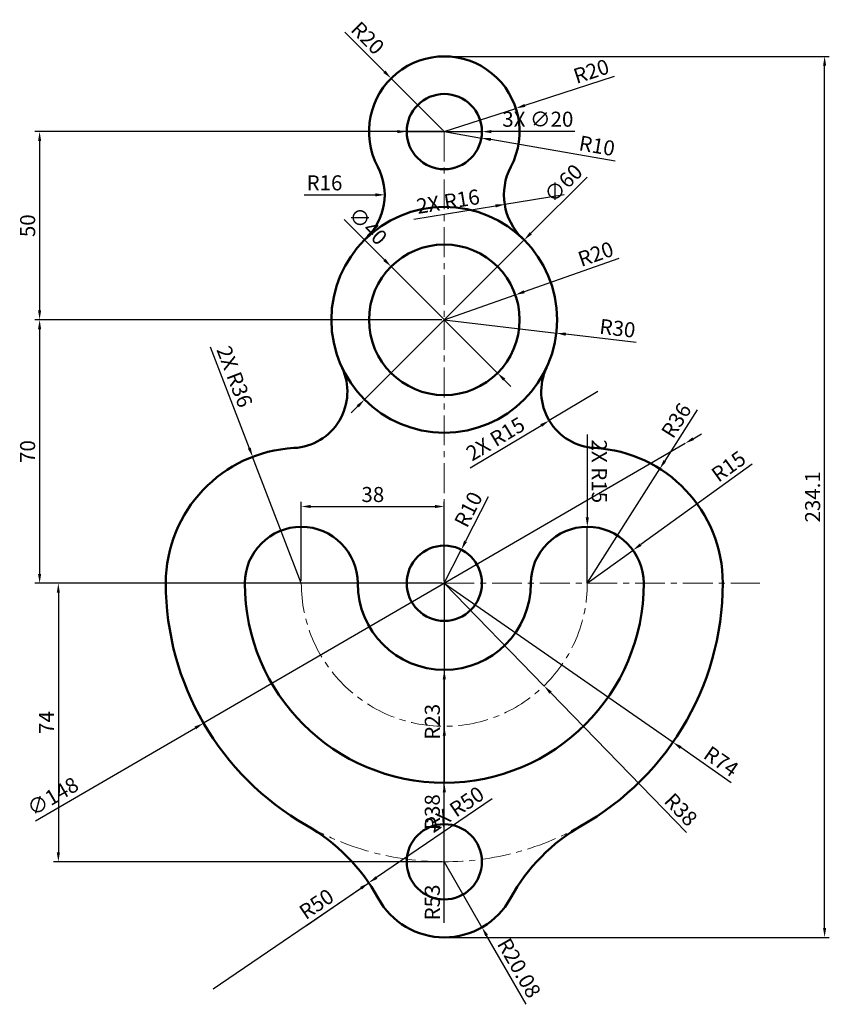
# Model space of a CAD drawing. Units: millimetres. Extents: x 2943 to 3158, y 1764 to 2026.
import ezdxf

# ---------------------------------------------------------------- set-up
doc = ezdxf.new("R2010")
doc.units = ezdxf.units.MM
doc.linetypes.add('CENTER', pattern=[50.8, 31.75, -6.35, 6.35, -6.35])
for name, color, linetype, lineweight in [('M-CNTR', 4, 'CENTER', 18), ('M-DIMS', 2, 'Continuous', 25), ('M-OUTL', 7, 'Continuous', 50)]:
    doc.layers.add(name, color=color, linetype=linetype, lineweight=lineweight)
doc.styles.get("Standard").update_dxf_attribs({"font": 'arial.ttf'})
doc.dimstyles.new('ISO-25', dxfattribs={"dimtxt": 4, "dimasz": 2.5, "dimexe": 1.25, "dimexo": 0.625, "dimtad": 1, "dimtxsty": 'Standard', "dimcen": 2.5, "dimadec": 0, "dimazin": 0, "dimtfac": 1, "dimtmove": 0, "dimatfit": 3, "dimfxl": 1, "dimarcsym": 0})

# ---------------------------------------------------------------- blocks, each defined once
blk = doc.blocks.new('*D1')
at = {"layer": 'Defpoints', "color": 0, "transparency": 16777216}
for p in [(3055.79, 1995.84), (2948.25, 1945.84), (3055.79, 1945.84)]:
    blk.add_point(p, dxfattribs=at)
at = {"layer": 'M-DIMS', "color": 0, "lineweight": -2, "transparency": 16777216}
for p, q in [((3055.16, 1995.84), (2947, 1995.84)), ((2948.25, 1993.34), (2948.25, 1948.34)), ((3055.16, 1945.84), (2947, 1945.84))]:
    blk.add_line(p, q, dxfattribs=at)
at = {"layer": 'M-DIMS', "color": 0, "transparency": 16777216}
for points in [[(2947.83, 1993.34), (2948.66, 1993.34), (2948.25, 1995.84)], [(2947.83, 1948.34), (2948.66, 1948.34), (2948.25, 1945.84)]]:
    blk.add_solid(points, dxfattribs=at)
at = {"layer": 'M-DIMS', "color": 0, "transparency": 16777216, "insert": (2945.58, 1970.84), "char_height": 4, "attachment_point": 5, "rotation": 90}
blk.add_mtext('50', dxfattribs=at)
blk = doc.blocks.new('*D2')
at = {"layer": 'Defpoints', "color": 0, "transparency": 16777216}
for p in [(3055.79, 1945.84), (2948.25, 1875.84), (3055.79, 1875.84)]:
    blk.add_point(p, dxfattribs=at)
at = {"layer": 'M-DIMS', "color": 0, "lineweight": -2, "transparency": 16777216}
for p, q in [((3055.16, 1945.84), (2947, 1945.84)), ((2948.25, 1943.34), (2948.25, 1878.34)), ((3055.16, 1875.84), (2947, 1875.84))]:
    blk.add_line(p, q, dxfattribs=at)
at = {"layer": 'M-DIMS', "color": 0, "transparency": 16777216}
for points in [[(2947.83, 1943.34), (2948.66, 1943.34), (2948.25, 1945.84)], [(2947.83, 1878.34), (2948.66, 1878.34), (2948.25, 1875.84)]]:
    blk.add_solid(points, dxfattribs=at)
at = {"layer": 'M-DIMS', "color": 0, "transparency": 16777216, "insert": (2945.58, 1910.84), "char_height": 4, "attachment_point": 5, "rotation": 90}
blk.add_mtext('70', dxfattribs=at)
blk = doc.blocks.new('*D3')
at = {"layer": 'Defpoints', "color": 0, "transparency": 16777216}
for p in [(3055.79, 1875.84), (2953.23, 1801.84), (3055.79, 1801.84)]:
    blk.add_point(p, dxfattribs=at)
at = {"layer": 'M-DIMS', "color": 0, "lineweight": -2, "transparency": 16777216}
for p, q in [((3055.16, 1875.84), (2951.98, 1875.84)), ((2953.23, 1873.34), (2953.23, 1804.34)), ((3055.16, 1801.84), (2951.98, 1801.84))]:
    blk.add_line(p, q, dxfattribs=at)
at = {"layer": 'M-DIMS', "color": 0, "transparency": 16777216}
for points in [[(2952.81, 1873.34), (2953.64, 1873.34), (2953.23, 1875.84)], [(2952.81, 1804.34), (2953.64, 1804.34), (2953.23, 1801.84)]]:
    blk.add_solid(points, dxfattribs=at)
at = {"layer": 'M-DIMS', "color": 0, "transparency": 16777216, "insert": (2950.6, 1838.84), "char_height": 4, "attachment_point": 5, "rotation": 90}
blk.add_mtext('74', dxfattribs=at)
blk = doc.blocks.new('*D4')
at = {"layer": 'Defpoints', "color": 0, "transparency": 16777216}
for p in [(3055.79, 1896.24), (3017.79, 1875.84), (3055.79, 1875.84)]:
    blk.add_point(p, dxfattribs=at)
at = {"layer": 'M-DIMS', "color": 0, "lineweight": -2, "transparency": 16777216}
for p, q in [((3017.79, 1876.47), (3017.79, 1897.49)), ((3055.79, 1876.47), (3055.79, 1897.49)), ((3020.29, 1896.24), (3053.29, 1896.24))]:
    blk.add_line(p, q, dxfattribs=at)
at = {"layer": 'M-DIMS', "color": 0, "transparency": 16777216}
for points in [[(3020.29, 1896.66), (3020.29, 1895.83), (3017.79, 1896.24)], [(3053.29, 1896.66), (3053.29, 1895.83), (3055.79, 1896.24)]]:
    blk.add_solid(points, dxfattribs=at)
at = {"layer": 'M-DIMS', "color": 0, "transparency": 16777216, "insert": (3036.79, 1898.91), "char_height": 4, "attachment_point": 5}
blk.add_mtext('38', dxfattribs=at)
blk = doc.blocks.new('*D5')
at = {"layer": 'Defpoints', "color": 0, "transparency": 16777216}
for p in [(3074.81, 2002.02), (3055.79, 1995.84)]:
    blk.add_point(p, dxfattribs=at)
at = {"layer": 'M-DIMS', "color": 0, "lineweight": -2, "transparency": 16777216}
for p, q in [((3100.96, 2010.52), (3077.19, 2002.79)), ((3055.79, 1995.84), (3074.81, 2002.02))]:
    blk.add_line(p, q, dxfattribs=at)
at = {"layer": 'M-DIMS', "color": 0, "transparency": 16777216}
blk.add_solid([(3077.06, 2003.19), (3077.32, 2002.4), (3074.81, 2002.02)], dxfattribs=at)
at = {"layer": 'M-DIMS', "color": 0, "transparency": 16777216, "insert": (3095, 2011.39), "char_height": 4, "attachment_point": 5, "rotation": 17.9978}
blk.add_mtext('R20', dxfattribs=at)
blk = doc.blocks.new('*D6')
at = {"layer": 'Defpoints', "color": 0, "transparency": 16777216}
for p in [(3055.79, 1995.84), (3065.64, 1994.14)]:
    blk.add_point(p, dxfattribs=at)
at = {"layer": 'M-DIMS', "color": 0, "lineweight": -2, "transparency": 16777216}
for p, q in [((3055.79, 1995.84), (3065.64, 1994.14)), ((3101.15, 1988.02), (3068.11, 1993.72))]:
    blk.add_line(p, q, dxfattribs=at)
at = {"layer": 'M-DIMS', "color": 0, "transparency": 16777216}
blk.add_solid([(3068.18, 1994.13), (3068.04, 1993.31), (3065.64, 1994.14)], dxfattribs=at)
at = {"layer": 'M-DIMS', "color": 0, "transparency": 16777216, "insert": (3096.28, 1991.57), "char_height": 4, "attachment_point": 5, "rotation": 350.2218}
blk.add_mtext('R10', dxfattribs=at)
blk = doc.blocks.new('*D7')
at = {"layer": 'Defpoints', "color": 0, "transparency": 16777216}
for p in [(3023.95, 1979.04), (3039.95, 1979.04)]:
    blk.add_point(p, dxfattribs=at)
at = {"layer": 'M-DIMS', "color": 0, "lineweight": -2, "transparency": 16777216}
blk.add_line((3018.55, 1979.04), (3037.45, 1979.04), dxfattribs=at)
at = {"layer": 'M-DIMS', "color": 0, "transparency": 16777216}
blk.add_solid([(3037.45, 1979.46), (3037.45, 1978.62), (3039.95, 1979.04)], dxfattribs=at)
at = {"layer": 'M-DIMS', "color": 0, "transparency": 16777216, "insert": (3023.95, 1981.71), "char_height": 4, "attachment_point": 5}
blk.add_mtext('R16', dxfattribs=at)
blk = doc.blocks.new('*D8')
at = {"layer": 'Defpoints', "color": 0, "transparency": 16777216}
for p in [(3060.31, 1884.76), (3055.79, 1875.84)]:
    blk.add_point(p, dxfattribs=at)
at = {"layer": 'M-DIMS', "color": 0, "lineweight": -2, "transparency": 16777216}
for p, q in [((3067.46, 1898.85), (3061.44, 1886.99)), ((3055.79, 1875.84), (3060.31, 1884.76))]:
    blk.add_line(p, q, dxfattribs=at)
at = {"layer": 'M-DIMS', "color": 0, "transparency": 16777216}
blk.add_solid([(3061.07, 1887.18), (3061.81, 1886.8), (3060.31, 1884.76)], dxfattribs=at)
at = {"layer": 'M-DIMS', "color": 0, "transparency": 16777216, "insert": (3062.64, 1895.24), "char_height": 4, "attachment_point": 5, "rotation": 63.1082}
blk.add_mtext('R10', dxfattribs=at)
blk = doc.blocks.new('*D9')
at = {"layer": 'Defpoints', "color": 0, "transparency": 16777216}
for p in [(3105.94, 1884.63), (3093.79, 1875.84)]:
    blk.add_point(p, dxfattribs=at)
at = {"layer": 'M-DIMS', "color": 0, "lineweight": -2, "transparency": 16777216}
for p, q in [((3137.58, 1907.51), (3107.97, 1886.1)), ((3093.79, 1875.84), (3105.94, 1884.63))]:
    blk.add_line(p, q, dxfattribs=at)
at = {"layer": 'M-DIMS', "color": 0, "transparency": 16777216}
blk.add_solid([(3107.73, 1886.43), (3108.21, 1885.76), (3105.94, 1884.63)], dxfattribs=at)
at = {"layer": 'M-DIMS', "color": 0, "transparency": 16777216, "insert": (3131.63, 1906.49), "char_height": 4, "attachment_point": 5, "rotation": 35.8697}
blk.add_mtext('R15', dxfattribs=at)
blk = doc.blocks.new('*D10')
at = {"layer": 'Defpoints', "color": 0, "transparency": 16777216}
for p in [(3113.05, 1906.25), (3093.79, 1875.84)]:
    blk.add_point(p, dxfattribs=at)
at = {"layer": 'M-DIMS', "color": 0, "lineweight": -2, "transparency": 16777216}
for p, q in [((3123.01, 1921.96), (3114.39, 1908.36)), ((3093.79, 1875.84), (3113.05, 1906.25))]:
    blk.add_line(p, q, dxfattribs=at)
at = {"layer": 'M-DIMS', "color": 0, "transparency": 16777216}
blk.add_solid([(3114.04, 1908.59), (3114.74, 1908.14), (3113.05, 1906.25)], dxfattribs=at)
at = {"layer": 'M-DIMS', "color": 0, "transparency": 16777216, "insert": (3117.86, 1918.82), "char_height": 4, "attachment_point": 5, "rotation": 57.646}
blk.add_mtext('R36', dxfattribs=at)
blk = doc.blocks.new('*D11')
at = {"layer": 'Defpoints', "color": 0, "transparency": 16777216}
for p in [(3074.66, 1952.46), (3055.79, 1945.84)]:
    blk.add_point(p, dxfattribs=at)
at = {"layer": 'M-DIMS', "color": 0, "lineweight": -2, "transparency": 16777216}
for p, q in [((3102.17, 1962.11), (3077.02, 1953.29)), ((3055.79, 1945.84), (3074.66, 1952.46))]:
    blk.add_line(p, q, dxfattribs=at)
at = {"layer": 'M-DIMS', "color": 0, "transparency": 16777216}
blk.add_solid([(3076.88, 1953.68), (3077.16, 1952.9), (3074.66, 1952.46)], dxfattribs=at)
at = {"layer": 'M-DIMS', "color": 0, "transparency": 16777216, "insert": (3096.19, 1962.84), "char_height": 4, "attachment_point": 5, "rotation": 19.3299}
blk.add_mtext('R20', dxfattribs=at)
blk = doc.blocks.new('*D12')
at = {"layer": 'Defpoints', "color": 0, "transparency": 16777216}
for p in [(3055.79, 1945.84), (3085.58, 1942.3)]:
    blk.add_point(p, dxfattribs=at)
at = {"layer": 'M-DIMS', "color": 0, "lineweight": -2, "transparency": 16777216}
for p, q in [((3055.79, 1945.84), (3085.58, 1942.3)), ((3106.79, 1939.78), (3088.06, 1942))]:
    blk.add_line(p, q, dxfattribs=at)
at = {"layer": 'M-DIMS', "color": 0, "transparency": 16777216}
blk.add_solid([(3088.11, 1942.42), (3088.01, 1941.59), (3085.58, 1942.3)], dxfattribs=at)
at = {"layer": 'M-DIMS', "color": 0, "transparency": 16777216, "insert": (3101.75, 1943.07), "char_height": 4, "attachment_point": 5, "rotation": 353.2204}
blk.add_mtext('R30', dxfattribs=at)
blk = doc.blocks.new('*D13')
at = {"layer": 'Defpoints', "color": 0, "transparency": 16777216}
for p in [(3055.79, 1875.84), (3082.27, 1848.59)]:
    blk.add_point(p, dxfattribs=at)
at = {"layer": 'M-DIMS', "color": 0, "lineweight": -2, "transparency": 16777216}
for p, q in [((3055.79, 1875.84), (3082.27, 1848.59)), ((3120.15, 1809.62), (3084.02, 1846.8))]:
    blk.add_line(p, q, dxfattribs=at)
at = {"layer": 'M-DIMS', "color": 0, "transparency": 16777216}
blk.add_solid([(3084.31, 1847.09), (3083.72, 1846.51), (3082.27, 1848.59)], dxfattribs=at)
at = {"layer": 'M-DIMS', "color": 0, "transparency": 16777216, "insert": (3118.29, 1815.36), "char_height": 4, "attachment_point": 5, "rotation": 314.1837}
blk.add_mtext('R38', dxfattribs=at)
blk = doc.blocks.new('*D14')
at = {"layer": 'Defpoints', "color": 0, "transparency": 16777216}
for p in [(3055.79, 1875.84), (3116.56, 1833.61)]:
    blk.add_point(p, dxfattribs=at)
at = {"layer": 'M-DIMS', "color": 0, "lineweight": -2, "transparency": 16777216}
for p, q in [((3055.79, 1875.84), (3116.56, 1833.61)), ((3132.02, 1822.86), (3118.61, 1832.18))]:
    blk.add_line(p, q, dxfattribs=at)
at = {"layer": 'M-DIMS', "color": 0, "transparency": 16777216}
blk.add_solid([(3118.85, 1832.53), (3118.37, 1831.84), (3116.56, 1833.61)], dxfattribs=at)
at = {"layer": 'M-DIMS', "color": 0, "transparency": 16777216, "insert": (3129.08, 1828.1), "char_height": 4, "attachment_point": 5, "rotation": 325.2015}
blk.add_mtext('R74', dxfattribs=at)
blk = doc.blocks.new('*D15')
at = {"layer": 'Defpoints', "color": 0, "transparency": 16777216}
for p in [(3035.71, 1796.23), (2994.35, 1768.13)]:
    blk.add_point(p, dxfattribs=at)
at = {"layer": 'M-DIMS', "color": 0, "lineweight": -2, "transparency": 16777216}
blk.add_line((3019.13, 1784.96), (3033.64, 1794.82), dxfattribs=at)
at = {"layer": 'M-DIMS', "color": 0, "transparency": 16777216}
blk.add_solid([(3033.41, 1795.17), (3033.88, 1794.48), (3035.71, 1796.23)], dxfattribs=at)
at = {"layer": 'M-DIMS', "color": 0, "transparency": 16777216, "insert": (3022.1, 1790.2), "char_height": 4, "attachment_point": 5, "rotation": 34.1854}
blk.add_mtext('R50', dxfattribs=at)
blk = doc.blocks.new('HOLE-D20')
blk.add_circle((10, 10), 10)
blk = doc.blocks.new('*D17')
at = {"layer": 'Defpoints', "color": 0, "transparency": 16777216}
for p in [(3055.79, 2015.84), (3156.85, 2015.84), (3055.79, 1781.76)]:
    blk.add_point(p, dxfattribs=at)
at = {"layer": 'M-DIMS', "color": 0, "lineweight": -2, "transparency": 16777216}
for p, q in [((3056.41, 2015.84), (3158.1, 2015.84)), ((3156.85, 1784.26), (3156.85, 2013.34)), ((3056.41, 1781.76), (3158.1, 1781.76))]:
    blk.add_line(p, q, dxfattribs=at)
at = {"layer": 'M-DIMS', "color": 0, "transparency": 16777216}
for points in [[(3156.43, 2013.34), (3157.26, 2013.34), (3156.85, 2015.84)], [(3156.43, 1784.26), (3157.26, 1784.26), (3156.85, 1781.76)]]:
    blk.add_solid(points, dxfattribs=at)
at = {"layer": 'M-DIMS', "color": 0, "transparency": 16777216, "insert": (3154.18, 1898.8), "char_height": 4, "attachment_point": 5, "rotation": 90}
blk.add_mtext('234.1', dxfattribs=at)
blk = doc.blocks.new('*D18')
at = {"layer": 'Defpoints', "color": 0, "transparency": 16777216}
for p in [(3041.65, 2009.98), (3055.79, 1995.84)]:
    blk.add_point(p, dxfattribs=at)
at = {"layer": 'M-DIMS', "color": 0, "lineweight": -2, "transparency": 16777216}
for p, q in [((3029.34, 2022.28), (3039.88, 2011.75)), ((3055.79, 1995.84), (3041.65, 2009.98))]:
    blk.add_line(p, q, dxfattribs=at)
at = {"layer": 'M-DIMS', "color": 0, "transparency": 16777216}
blk.add_solid([(3040.17, 2012.05), (3039.58, 2011.46), (3041.65, 2009.98)], dxfattribs=at)
at = {"layer": 'M-DIMS', "color": 0, "transparency": 16777216, "insert": (3035.05, 2020.35), "char_height": 4, "attachment_point": 5, "rotation": 315.0007}
blk.add_mtext('R20', dxfattribs=at)
blk = doc.blocks.new('*D19')
at = {"layer": 'Defpoints', "color": 0, "transparency": 16777216}
for p in [(3045.79, 1995.84), (3065.79, 1995.84)]:
    blk.add_point(p, dxfattribs=at)
at = {"layer": 'M-DIMS', "color": 0, "lineweight": -2, "transparency": 16777216}
for p, q in [((3043.29, 1995.84), (3040.79, 1995.84)), ((3045.79, 1995.84), (3065.79, 1995.84)), ((3090.49, 1995.84), (3068.29, 1995.84))]:
    blk.add_line(p, q, dxfattribs=at)
at = {"layer": 'M-DIMS', "color": 0, "transparency": 16777216}
for points in [[(3043.29, 1996.26), (3043.29, 1995.42), (3045.79, 1995.84)], [(3068.29, 1996.26), (3068.29, 1995.42), (3065.79, 1995.84)]]:
    blk.add_solid(points, dxfattribs=at)
at = {"layer": 'M-DIMS', "color": 0, "transparency": 16777216, "insert": (3080.64, 1998.62), "char_height": 4, "attachment_point": 5, "rotation": 359.9986}
blk.add_mtext('3X ∅20', dxfattribs=at)
blk = doc.blocks.new('*D20')
at = {"layer": 'Defpoints', "color": 0, "transparency": 16777216}
for p in [(3087.63, 1979.04), (3071.83, 1976.49)]:
    blk.add_point(p, dxfattribs=at)
at = {"layer": 'M-DIMS', "color": 0, "lineweight": -2, "transparency": 16777216}
for p, q in [((3087.63, 1979.04), (3071.83, 1976.49)), ((3047.68, 1972.58), (3069.37, 1976.09))]:
    blk.add_line(p, q, dxfattribs=at)
at = {"layer": 'M-DIMS', "color": 0, "transparency": 16777216}
blk.add_solid([(3069.3, 1976.5), (3069.43, 1975.68), (3071.83, 1976.49)], dxfattribs=at)
at = {"layer": 'M-DIMS', "color": 0, "transparency": 16777216, "insert": (3056.86, 1976.77), "char_height": 4, "attachment_point": 5, "rotation": 9.1897}
blk.add_mtext('2X R16', dxfattribs=at)
blk = doc.blocks.new('*D21')
at = {"layer": 'Defpoints', "color": 0, "transparency": 16777216}
for p in [(3077, 1967.05), (3034.57, 1924.63)]:
    blk.add_point(p, dxfattribs=at)
at = {"layer": 'M-DIMS', "color": 0, "lineweight": -2, "transparency": 16777216}
for p, q in [((3093.73, 1983.78), (3078.77, 1968.82)), ((3034.57, 1924.63), (3077, 1967.05)), ((3032.81, 1922.86), (3031.04, 1921.09))]:
    blk.add_line(p, q, dxfattribs=at)
at = {"layer": 'M-DIMS', "color": 0, "transparency": 16777216}
for points in [[(3078.48, 1969.12), (3079.07, 1968.53), (3077, 1967.05)], [(3032.51, 1923.16), (3033.1, 1922.57), (3034.57, 1924.63)]]:
    blk.add_solid(points, dxfattribs=at)
at = {"layer": 'M-DIMS', "color": 0, "transparency": 16777216, "insert": (3087.77, 1981.75), "char_height": 4, "attachment_point": 5, "rotation": 44.9971}
blk.add_mtext('∅60', dxfattribs=at)
blk = doc.blocks.new('*D22')
at = {"layer": 'Defpoints', "color": 0, "transparency": 16777216}
for p in [(3041.65, 1959.98), (3069.93, 1931.7)]:
    blk.add_point(p, dxfattribs=at)
at = {"layer": 'M-DIMS', "color": 0, "lineweight": -2, "transparency": 16777216}
for p, q in [((3029.16, 1972.47), (3039.88, 1961.75)), ((3069.93, 1931.7), (3041.65, 1959.98)), ((3071.7, 1929.93), (3073.47, 1928.16))]:
    blk.add_line(p, q, dxfattribs=at)
at = {"layer": 'M-DIMS', "color": 0, "transparency": 16777216}
for points in [[(3040.17, 1962.05), (3039.58, 1961.46), (3041.65, 1959.98)], [(3071.99, 1930.23), (3071.4, 1929.64), (3069.93, 1931.7)]]:
    blk.add_solid(points, dxfattribs=at)
at = {"layer": 'M-DIMS', "color": 0, "transparency": 16777216, "insert": (3035.13, 1970.43), "char_height": 4, "attachment_point": 5, "rotation": 315.0007}
blk.add_mtext('∅40', dxfattribs=at)
blk = doc.blocks.new('*D23')
at = {"layer": 'Defpoints', "color": 0, "transparency": 16777216}
for p in [(3096.55, 1926.77), (3083.68, 1919.06)]:
    blk.add_point(p, dxfattribs=at)
at = {"layer": 'M-DIMS', "color": 0, "lineweight": -2, "transparency": 16777216}
for p, q in [((3096.55, 1926.77), (3083.68, 1919.06)), ((3062.66, 1906.47), (3081.53, 1917.78))]:
    blk.add_line(p, q, dxfattribs=at)
at = {"layer": 'M-DIMS', "color": 0, "transparency": 16777216}
blk.add_solid([(3081.32, 1918.13), (3081.75, 1917.42), (3083.68, 1919.06)], dxfattribs=at)
at = {"layer": 'M-DIMS', "color": 0, "transparency": 16777216, "insert": (3069.65, 1913.77), "char_height": 4, "attachment_point": 5, "rotation": 30.9114}
blk.add_mtext('2X R15', dxfattribs=at)
blk = doc.blocks.new('*D24')
at = {"layer": 'Defpoints', "color": 0, "transparency": 16777216}
for p in [(3004.86, 1909.44), (3017.79, 1875.84)]:
    blk.add_point(p, dxfattribs=at)
at = {"layer": 'M-DIMS', "color": 0, "lineweight": -2, "transparency": 16777216}
for p, q in [((2993.61, 1938.69), (3003.97, 1911.77)), ((3017.79, 1875.84), (3004.86, 1909.44))]:
    blk.add_line(p, q, dxfattribs=at)
at = {"layer": 'M-DIMS', "color": 0, "transparency": 16777216}
blk.add_solid([(3004.35, 1911.92), (3003.58, 1911.62), (3004.86, 1909.44)], dxfattribs=at)
at = {"layer": 'M-DIMS', "color": 0, "transparency": 16777216, "insert": (2999.6, 1930.56), "char_height": 4, "attachment_point": 5, "rotation": 291.0414}
blk.add_mtext('2X R36', dxfattribs=at)
blk = doc.blocks.new('*D25')
at = {"layer": 'Defpoints', "color": 0, "transparency": 16777216}
for p in [(3093.79, 1890.84), (3093.79, 1875.84)]:
    blk.add_point(p, dxfattribs=at)
at = {"layer": 'M-DIMS', "color": 0, "lineweight": -2, "transparency": 16777216}
for p, q in [((3093.79, 1915.34), (3093.79, 1893.34)), ((3093.79, 1875.84), (3093.79, 1890.84))]:
    blk.add_line(p, q, dxfattribs=at)
at = {"layer": 'M-DIMS', "color": 0, "transparency": 16777216}
blk.add_solid([(3094.21, 1893.34), (3093.37, 1893.34), (3093.79, 1890.84)], dxfattribs=at)
at = {"layer": 'M-DIMS', "color": 0, "transparency": 16777216, "insert": (3096.46, 1905.59), "char_height": 4, "attachment_point": 5, "rotation": 270.0003}
blk.add_mtext('2X R15', dxfattribs=at)
blk = doc.blocks.new('*D26')
at = {"layer": 'Defpoints', "color": 0, "transparency": 16777216}
for p in [(3119.78, 1913.01), (2991.8, 1838.67)]:
    blk.add_point(p, dxfattribs=at)
at = {"layer": 'M-DIMS', "color": 0, "lineweight": -2, "transparency": 16777216}
for p, q in [((3121.94, 1914.26), (3124.1, 1915.52)), ((3119.78, 1913.01), (2991.8, 1838.67)), ((2947.16, 1812.75), (2989.64, 1837.42))]:
    blk.add_line(p, q, dxfattribs=at)
at = {"layer": 'M-DIMS', "color": 0, "transparency": 16777216}
for points in [[(3121.73, 1914.62), (3122.15, 1913.9), (3119.78, 1913.01)], [(2989.43, 1837.78), (2989.85, 1837.06), (2991.8, 1838.67)]]:
    blk.add_solid(points, dxfattribs=at)
at = {"layer": 'M-DIMS', "color": 0, "transparency": 16777216, "insert": (2952.01, 1818.78), "char_height": 4, "attachment_point": 5, "rotation": 30.1496}
blk.add_mtext('∅148', dxfattribs=at)
blk = doc.blocks.new('*D27')
at = {"layer": 'Defpoints', "color": 0, "transparency": 16777216}
for p in [(3055.79, 1875.84), (3055.79, 1822.84)]:
    blk.add_point(p, dxfattribs=at)
at = {"layer": 'M-DIMS', "color": 0, "lineweight": -2, "transparency": 16777216}
for p, q in [((3055.79, 1875.84), (3055.79, 1822.84)), ((3055.79, 1785.64), (3055.79, 1820.34))]:
    blk.add_line(p, q, dxfattribs=at)
at = {"layer": 'M-DIMS', "color": 0, "transparency": 16777216}
blk.add_solid([(3055.37, 1820.34), (3056.21, 1820.34), (3055.79, 1822.84)], dxfattribs=at)
at = {"layer": 'M-DIMS', "color": 0, "transparency": 16777216, "insert": (3053.12, 1791.04), "char_height": 4, "attachment_point": 5, "rotation": 89.9999}
blk.add_mtext('R53', dxfattribs=at)
blk = doc.blocks.new('*D28')
at = {"layer": 'Defpoints', "color": 0, "transparency": 16777216}
for p in [(3055.79, 1875.84), (3055.79, 1837.84)]:
    blk.add_point(p, dxfattribs=at)
at = {"layer": 'M-DIMS', "color": 0, "lineweight": -2, "transparency": 16777216}
for p, q in [((3055.79, 1875.84), (3055.79, 1837.84)), ((3055.79, 1809.63), (3055.79, 1835.34))]:
    blk.add_line(p, q, dxfattribs=at)
at = {"layer": 'M-DIMS', "color": 0, "transparency": 16777216}
blk.add_solid([(3055.37, 1835.34), (3056.21, 1835.34), (3055.79, 1837.84)], dxfattribs=at)
at = {"layer": 'M-DIMS', "color": 0, "transparency": 16777216, "insert": (3053.12, 1815.04), "char_height": 4, "attachment_point": 5, "rotation": 89.9999}
blk.add_mtext('R38', dxfattribs=at)
blk = doc.blocks.new('*D29')
at = {"layer": 'Defpoints', "color": 0, "transparency": 16777216}
for p in [(3055.79, 1875.84), (3055.79, 1852.84)]:
    blk.add_point(p, dxfattribs=at)
at = {"layer": 'M-DIMS', "color": 0, "lineweight": -2, "transparency": 16777216}
for p, q in [((3055.79, 1875.84), (3055.79, 1852.84)), ((3055.79, 1833.64), (3055.79, 1850.34))]:
    blk.add_line(p, q, dxfattribs=at)
at = {"layer": 'M-DIMS', "color": 0, "transparency": 16777216}
blk.add_solid([(3055.37, 1850.34), (3056.21, 1850.34), (3055.79, 1852.84)], dxfattribs=at)
at = {"layer": 'M-DIMS', "color": 0, "transparency": 16777216, "insert": (3053.12, 1839.04), "char_height": 4, "attachment_point": 5, "rotation": 89.9998}
blk.add_mtext('R23', dxfattribs=at)
blk = doc.blocks.new('*D30')
at = {"layer": 'Defpoints', "color": 0, "transparency": 16777216}
for p in [(3035.69, 1796.25), (2994.35, 1768.13)]:
    blk.add_point(p, dxfattribs=at)
at = {"layer": 'M-DIMS', "color": 0, "lineweight": -2, "transparency": 16777216}
for p, q in [((3068.54, 1818.6), (3037.76, 1797.66)), ((2994.35, 1768.13), (3035.69, 1796.25))]:
    blk.add_line(p, q, dxfattribs=at)
at = {"layer": 'M-DIMS', "color": 0, "transparency": 16777216}
blk.add_solid([(3037.53, 1798), (3038, 1797.31), (3035.69, 1796.25)], dxfattribs=at)
at = {"layer": 'M-DIMS', "color": 0, "transparency": 16777216, "insert": (3059, 1815.33), "char_height": 4, "attachment_point": 5, "rotation": 34.2234}
blk.add_mtext('2X R50', dxfattribs=at)
blk = doc.blocks.new('*D31')
at = {"layer": 'Defpoints', "color": 0, "transparency": 16777216}
for p in [(3055.79, 1801.84), (3065.79, 1784.43)]:
    blk.add_point(p, dxfattribs=at)
at = {"layer": 'M-DIMS', "color": 0, "lineweight": -2, "transparency": 16777216}
for p, q in [((3055.79, 1801.84), (3065.79, 1784.43)), ((3077.53, 1763.98), (3067.03, 1782.26))]:
    blk.add_line(p, q, dxfattribs=at)
at = {"layer": 'M-DIMS', "color": 0, "transparency": 16777216}
blk.add_solid([(3067.4, 1782.47), (3066.67, 1782.05), (3065.79, 1784.43)], dxfattribs=at)
at = {"layer": 'M-DIMS', "color": 0, "transparency": 16777216, "insert": (3075.22, 1773.37), "char_height": 4, "attachment_point": 5, "rotation": 299.8704}
blk.add_mtext('R20.08', dxfattribs=at)

msp = doc.modelspace()

# ---------------------------------------------------------------- linework, layer by layer
at = {"layer": 'M-CNTR', "ltscale": 0.25}
for p, q in [((3055.789, 1995.841), (3055.789, 1945.841)), ((3055.789, 1945.841), (3055.789, 1801.841)), ((3017.789, 1875.841), (2976.185, 1875.841)), ((3055.789, 1875.841), (3017.789, 1875.841)), ((3055.789, 1875.841), (3093.789, 1875.841)), ((3093.789, 1875.841), (3139.646, 1875.841))]:
    msp.add_line(p, q, dxfattribs=at)
for radius, start, end in [(38, 180, 0), (74, 238.24465, 299.7005)]:
    msp.add_arc((3055.789, 1875.841), radius, start, end, dxfattribs=at)
at = {"layer": 'M-OUTL'}
msp.add_line((3089.611, 1810.023), (3089.698, 1809.871), dxfattribs=at)
for radius in [30, 20]:
    msp.add_circle((3055.789, 1945.841), radius, dxfattribs=at)
for centre, radius, start, end in [((3055.789, 1995.841), 20, 332.18186, 207.81814), ((3023.949, 1979.041), 16, 313.80175, 27.81814), ((3087.629, 1979.041), 16, 152.18186, 226.19825), ((3015.032, 1926.767), 15, 273.09922, 25.07978), ((3096.546, 1926.767), 15, 154.92022, 266.90078), ((3017.789, 1875.841), 36, 93.09922, 180), ((3093.789, 1875.841), 36, 360, 86.90078), ((3017.789, 1875.841), 15, 0, 180), ((3093.789, 1875.841), 15, 0, 180), ((3055.789, 1875.841), 74, 180, 240.2995), ((3055.789, 1875.841), 53, 180, 0), ((3055.789, 1875.841), 23, 180, 0), ((3055.789, 1875.841), 74, 297.19677, 360), ((2994.351, 1768.131), 50, 28.75275, 60.2995), ((3117.227, 1768.131), 50, 119.7005, 151.24725), ((3055.789, 1801.841), 20.078, 208.75275, 331.24725)]:
    msp.add_arc(centre, radius, start, end, dxfattribs=at)

# ---------------------------------------------------------------- block references
for p in [(3045.789, 1985.841), (3045.789, 1865.841), (3045.789, 1791.841)]:
    msp.add_blockref('HOLE-D20', p, dxfattribs=at)

# ---------------------------------------------------------------- dimensions: what is measured, and where the dimension line sits
at = {"layer": 'M-DIMS'}
for center, mpoint, override, picture, middle in [((3055.789, 1995.841), (3041.647, 2009.983), {"dimdec": 0, "dimlfac": 1, "dimrnd": 0, "dimzin": 0, "dimdsep": 46, "dimlunit": 2}, '*D18', (3033.161, 2018.468)), ((3055.789, 1995.841), (3074.81, 2002.021), {"dimclrd": 0, "dimclre": 0, "dimclrt": 0}, '*D5', (3095.828, 2008.849)), ((3055.789, 1995.841), (3065.644, 1994.143), {"dimclrd": 0, "dimclre": 0, "dimclrt": 0}, '*D6', (3095.828, 1988.941)), ((3023.949, 1979.041), (3039.949, 1979.041), {"dimclrd": 0, "dimclre": 0, "dimclrt": 0}, '*D7', (3023.949, 1979.041)), ((3055.789, 1945.841), (3074.662, 1952.461), {"dimclrd": 0, "dimclre": 0, "dimclrt": 0}, '*D11', (3097.074, 1960.323)), ((3055.789, 1945.841), (3085.579, 1942.3), {"dimclrd": 0, "dimclre": 0, "dimclrt": 0}, '*D12', (3101.433, 1940.415)), ((3093.789, 1875.841), (3113.054, 1906.253), {"dimclrd": 0, "dimclre": 0, "dimclrt": 0}, '*D10', (3120.114, 1917.396)), ((3093.789, 1875.841), (3105.944, 1884.63), {"dimclrd": 0, "dimclre": 0, "dimclrt": 0}, '*D9', (3133.191, 1904.332)), ((3055.789, 1875.841), (3055.789, 1822.841), {"dimdec": 0, "dimlfac": 1, "dimrnd": 0, "dimzin": 0, "dimdsep": 46, "dimlunit": 2}, '*D27', (3055.789, 1791.041)), ((3055.789, 1875.841), (3055.789, 1837.841), {"dimdec": 0, "dimlfac": 1, "dimrnd": 0, "dimzin": 0, "dimdsep": 46, "dimlunit": 2}, '*D28', (3055.789, 1815.041)), ((3055.789, 1875.841), (3055.789, 1852.841), {"dimdec": 0, "dimlfac": 1, "dimrnd": 0, "dimzin": 0, "dimdsep": 46, "dimlunit": 2}, '*D29', (3055.789, 1839.041)), ((3055.789, 1875.841), (3082.274, 1848.591), {"dimclrd": 0, "dimclre": 0, "dimclrt": 0}, '*D13', (3116.378, 1813.501)), ((3055.789, 1875.841), (3116.555, 1833.61), {"dimclrd": 0, "dimclre": 0, "dimclrt": 0}, '*D14', (3127.586, 1825.944)), ((2994.351, 1768.131), (3035.712, 1796.225), {"dimclrd": 0, "dimclre": 0, "dimclrt": 0}, '*D15', (3023.594, 1787.994))]:
    dim = msp.add_radius_dim(center=center, mpoint=mpoint, dimstyle='ISO-25', override=override, dxfattribs=at)
    dim.commit()
    dim.dimension.update_dxf_attribs({"geometry": picture, "text_midpoint": middle, "dimtype": 164})
for base, p1, p2, override, picture, middle in [((3156.846, 2015.841), (3055.789, 1781.763), (3055.789, 2015.841), {"dimdec": 1, "dimlfac": 1, "dimrnd": 0, "dimzin": 0, "dimdsep": 46, "dimlunit": 2}, '*D17', (3154.178, 1898.802)), ((2948.246, 1945.841), (3055.789, 1995.841), (3055.789, 1945.841), {"dimclrd": 0, "dimclre": 0, "dimclrt": 0}, '*D1', (2945.579, 1970.841)), ((2948.246, 1875.841), (3055.789, 1945.841), (3055.789, 1875.841), {"dimclrd": 0, "dimclre": 0, "dimclrt": 0}, '*D2', (2945.579, 1910.841)), ((2953.228, 1801.841), (3055.789, 1875.841), (3055.789, 1801.841), {"dimclrd": 0, "dimclre": 0, "dimclrt": 0}, '*D3', (2950.603, 1838.841))]:
    dim = msp.add_linear_dim(base=base, p1=p1, p2=p2, angle=90, dimstyle='ISO-25', override=override, dxfattribs=at)
    dim.commit()
    dim.dimension.update_dxf_attribs({"geometry": picture, "text_midpoint": middle})
dim = msp.add_diameter_dim_2p(p1=(3045.789, 1995.842), p2=(3065.789, 1995.841), text='3X <>', dimstyle='ISO-25', override={"dimdec": 0, "dimlfac": 1, "dimrnd": 0, "dimzin": 0, "dimdsep": 46, "dimlunit": 2}, dxfattribs=at)
dim.commit()
dim.dimension.update_dxf_attribs({"geometry": '*D19', "text_midpoint": (3080.638, 1995.841)})
for p1, p2, picture, middle in [((3034.575, 1924.629), (3077.003, 1967.053), '*D21', (3089.732, 1979.781)), ((3069.931, 1931.699), (3041.647, 1959.983), '*D22', (3033.161, 1968.468)), ((3119.778, 1913.008), (2991.8, 1838.674), '*D26', (2953.407, 1816.374))]:
    dim = msp.add_diameter_dim_2p(p1=p1, p2=p2, dimstyle='ISO-25', override={"dimdec": 0, "dimlfac": 1, "dimrnd": 0, "dimzin": 0, "dimdsep": 46, "dimlunit": 2}, dxfattribs=at)
    dim.commit()
    dim.dimension.update_dxf_attribs({"geometry": picture, "text_midpoint": middle, "dimtype": 163})
for center, mpoint, picture, middle in [((3087.629, 1979.041), (3071.834, 1976.486), '*D20', (3056.863, 1976.766)), ((3096.546, 1926.767), (3083.677, 1919.061), '*D23', (3069.651, 1913.772)), ((3093.789, 1875.841), (3093.789, 1890.841), '*D25', (3096.456, 1905.592))]:
    dim = msp.add_radius_dim(center=center, mpoint=mpoint, text='2X <>', dimstyle='ISO-25', override={"dimdec": 0, "dimlfac": 1, "dimrnd": 0, "dimzin": 0, "dimdsep": 46, "dimlunit": 2}, dxfattribs=at)
    dim.commit()
    dim.dimension.update_dxf_attribs({"geometry": picture, "text_midpoint": middle})
for center, mpoint, picture, middle in [((3017.789, 1875.841), (3004.864, 1909.441), '*D24', (2997.108, 1929.601)), ((2994.351, 1768.131), (3035.694, 1796.253), '*D30', (3060.499, 1813.125))]:
    dim = msp.add_radius_dim(center=center, mpoint=mpoint, text='2X <>', dimstyle='ISO-25', override={"dimdec": 0, "dimlfac": 1, "dimrnd": 0, "dimzin": 0, "dimdsep": 46, "dimlunit": 2}, dxfattribs=at)
    dim.commit()
    dim.dimension.update_dxf_attribs({"geometry": picture, "text_midpoint": middle, "dimtype": 164})
dim = msp.add_linear_dim(base=(3055.789, 1896.244), p1=(3017.789, 1875.841), p2=(3055.789, 1875.841), dimstyle='ISO-25', override={"dimclrd": 0, "dimclre": 0, "dimclrt": 0}, dxfattribs=at)
dim.commit()
dim.dimension.update_dxf_attribs({"geometry": '*D4', "text_midpoint": (3036.789, 1898.913)})
for center, mpoint, override, picture, middle in [((3055.789, 1875.841), (3060.312, 1884.76), {"dimclrd": 0, "dimclre": 0, "dimclrt": 0}, '*D8', (3062.636, 1895.239)), ((3055.789, 1801.841), (3065.789, 1784.43), {"dimdec": 2, "dimlfac": 1, "dimrnd": 0, "dimzin": 0, "dimdsep": 46, "dimlunit": 2}, '*D31', (3075.22, 1773.365))]:
    dim = msp.add_radius_dim(center=center, mpoint=mpoint, dimstyle='ISO-25', override=override, dxfattribs=at)
    dim.commit()
    dim.dimension.update_dxf_attribs({"geometry": picture, "text_midpoint": middle})

doc.saveas('drawing.dxf')
